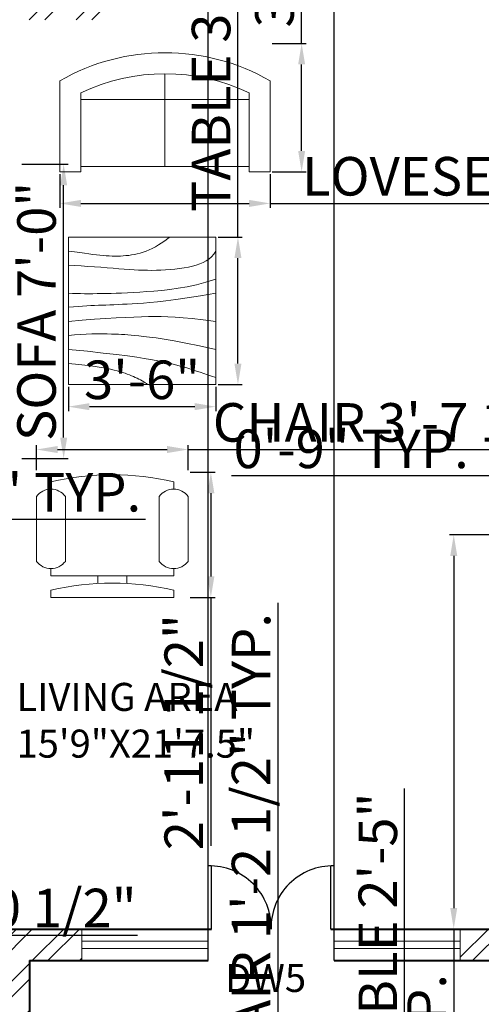
# Model space of a CAD drawing. Units: inches. Extents: x 2069 to 3028, y 691 to 1726.
# Tile 5 of 10: x 2481 to 2613, y 1044 to 1325. Entities that reach past the tile are written whole.
import ezdxf

# ---------------------------------------------------------------- set-up
doc = ezdxf.new("R2010")
doc.units = ezdxf.units.IN
for name, color, linetype, lineweight in [('A-ANNO-DIMS', 2, 'Continuous', 18), ('A-DOOR', 3, 'Continuous', 25), ('A-FURN', 8, 'Continuous', 18), ('A-GLAZ', 4, 'Continuous', 20), ('A-WALL', 7, 'Continuous', 40)]:
    doc.layers.add(name, color=color, linetype=linetype, lineweight=lineweight)
for name, color, linetype, lineweight, true_color in [('A-ANNO-TEXT', 11, 'Continuous', 18, 0xf27172), ('A-AREA-IDEN', 11, 'Continuous', 25, 0xf27172), ('A-WALL-PATT', 143, 'Continuous', 13, 0x7aafdf)]:
    doc.layers.add(name, color=color, linetype=linetype, lineweight=lineweight, true_color=true_color)
doc.styles.get("Standard").update_dxf_attribs({"font": 'arial.ttf'})
doc.dimstyles.new('ISO-25', dxfattribs={"dimtxt": 11, "dimasz": 6, "dimexe": 1.25, "dimexo": 0.625, "dimtad": 1, "dimlunit": 3, "dimtxsty": 'Standard', "dimcen": 2.5, "dimclrd": 3, "dimclre": 5, "dimclrt": 6, "dimadec": 0, "dimazin": 0, "dimtfac": 1, "dimtmove": 0, "dimatfit": 3, "dimfxl": 1, "dimarcsym": 0})

# ---------------------------------------------------------------- blocks, each defined once
blk = doc.blocks.new('Sofa - Roundback Loveseat 5 ft.')
for p, q in [((0, -32.44198), (0, -5.99998)), ((-24, -33.99998), (-24, -11.46958)), ((-23.9998, -13.38178), (23.99986, -13.38178)), ((24.00004, -33.99998), (24.00004, -11.46958)), ((-24, -32.44198), (24.00004, -32.44198))]:
    blk.add_line(p, q)
for points in [[(-24, -33.99998), (-30, -33.99998), (-30, -7.99998)], [(30.00004, -7.99998), (30.00004, -33.99998), (24.00004, -33.99998)]]:
    blk.add_lwpolyline(points)
for centre, radius, start, end in [((0, -60.24998), 60.24998, 60.13715, 119.8628), ((0, -61.38438), 55.38444, 64.32083, 115.6792)]:
    blk.add_arc(centre, radius, start, end)
blk = doc.blocks.new('Chair - Desk')
for p, q in [((-8.5, 0), (-8.5, -1)), ((-8.5, 0), (8.5, 0)), ((8.5, 0), (8.5, -1)), ((-2, -3), (-2, -1.9355)), ((2, -1.9576), (2, -3)), ((-8.5, -3), (-8.5, -4)), ((-8.5, -3), (8.5, -3)), ((8.5, -3), (8.5, -4)), ((-10.5, -5), (-10.5, -14)), ((-6.5, -14), (-6.5, -5)), ((6.5, -5), (6.5, -14)), ((10.5, -14), (10.5, -5)), ((-8.5, -15), (-8.5, -16)), ((8.5, -15), (8.5, -16))]:
    blk.add_line(p, q)
for centre, radius, start, end in [((0, 34.625), 36.625, 256.5803, 283.4197), ((-8.5, -6.5), 2.5, 36.8699, 143.1301), ((8.5, -6.5), 2.5, 36.8699, 143.1301), ((-8.5, -12.5), 2.5, 216.8699, 323.1301), ((8.5, -12.5), 2.5, 216.8699, 323.1301), ((0, 19.625), 36.625, 256.5803, 283.4197)]:
    blk.add_arc(centre, radius, start, end)
blk = doc.blocks.new('Table - Square Woodgrain 42 x 42 in.')
blk.add_line((0, -42), (42, -42))
for points in [[(0, -4), (1.704, -4.2172), (3.2358, -4.4188), (4.615, -4.604), (5.8615, -4.7721), (6.9951, -4.9224), (8.0357, -5.0541), (9.0031, -5.1667), (9.9171, -5.2594), (10.7951, -5.3316), (11.6445, -5.3836), (12.4702, -5.4157), (13.277, -5.4283), (14.0698, -5.4217), (14.8535, -5.3964), (15.6331, -5.3526), (16.4133, -5.2908), (17.1986, -5.2103), (17.9913, -5.1062), (18.793, -4.9727), (19.6056, -4.8038), (20.4307, -4.5937), (21.2701, -4.3365), (22.1256, -4.0262), (22.9989, -3.6571), (23.888, -3.2272), (24.7756, -2.7516), (25.6408, -2.2491), (26.4624, -1.7387), (27.2195, -1.2395), (27.891, -0.7703), (28.456, -0.3501), (28.8934, 0.002)], [(0, -42), (0, 0), (42, 0), (42, -42)], [(0, -8), (1.8203, -8.1001), (3.6741, -8.2149), (5.5411, -8.3408), (7.4011, -8.4741), (9.2339, -8.6112), (11.0193, -8.7484), (12.7371, -8.8821), (14.3671, -9.0086), (15.8954, -9.1246), (17.3337, -9.2278), (18.6997, -9.3159), (20.0116, -9.387), (21.2871, -9.4389), (22.5442, -9.4696), (23.8008, -9.477), (25.0749, -9.459), (26.3791, -9.4137), (27.7049, -9.3403), (29.0383, -9.2382), (30.3655, -9.1068), (31.6728, -8.9455), (32.9461, -8.7535), (34.1717, -8.5304), (35.3358, -8.2756), (36.4268, -7.9863), (37.443, -7.6521), (38.3849, -7.2603), (39.253, -6.7986), (40.048, -6.2542), (40.7705, -5.6147), (41.421, -4.8674), (42, -4)], [(42, -12), (39.1784, -12.8621), (36.4519, -13.5654), (33.8246, -14.1294), (31.3004, -14.5731), (28.8832, -14.9161), (26.577, -15.1775), (24.3858, -15.3768), (22.3136, -15.5332), (20.3622, -15.6632), (18.5254, -15.7718), (16.7947, -15.8612), (15.1618, -15.9338), (13.6183, -15.9916), (12.1558, -16.0369), (10.7659, -16.0718), (9.4403, -16.0987), (8.1703, -16.1191), (6.9461, -16.1325), (5.7577, -16.1377), (4.595, -16.1335), (3.4479, -16.1188), (2.3064, -16.0924), (1.1604, -16.0532), (0, -16)], [(42, -16), (37.6529, -16.7365), (33.8802, -17.329), (30.6179, -17.7961), (27.8015, -18.1561), (25.3668, -18.4275), (23.2497, -18.6288), (21.3859, -18.7785), (19.7111, -18.8949), (18.1693, -18.9939), (16.7375, -19.0795), (15.401, -19.1534), (14.1449, -19.217), (12.9544, -19.2717), (11.8148, -19.3191), (10.7113, -19.3606), (9.6291, -19.3976), (8.5534, -19.4323), (7.47, -19.4689), (6.3643, -19.5122), (5.222, -19.5672), (4.0288, -19.6386), (2.7703, -19.7313), (1.4321, -19.8501), (0, -20)], [(0, -24), (3.9243, -23.6805), (7.4766, -23.4138), (10.6891, -23.1954), (13.5943, -23.0205), (16.2247, -22.8847), (18.6125, -22.7832), (20.7903, -22.7116), (22.7903, -22.6651), (24.6563, -22.642), (26.4764, -22.6507), (28.35, -22.7024), (30.3766, -22.8084), (32.6555, -22.98), (35.2861, -23.2283), (38.3678, -23.5645), (42, -24)], [(42, -32), (37.392, -31.017), (33.4585, -30.2231), (30.1291, -29.5949), (27.3334, -29.109), (25.0009, -28.742), (23.0612, -28.4707), (21.4439, -28.2716), (20.0786, -28.1215), (18.8998, -28.0002), (17.8609, -27.9014), (16.9206, -27.8219), (16.0371, -27.7588), (15.1691, -27.709), (14.2748, -27.6693), (13.3128, -27.6368), (12.2415, -27.6083), (11.0295, -27.5824), (9.6867, -27.5643), (8.233, -27.5608), (6.6884, -27.5787), (5.0728, -27.6248), (3.4062, -27.7058), (1.7086, -27.8286), (0, -28)], [(0, -32), (5.4026, -32.5358), (9.9494, -33.019), (13.7424, -33.4553), (16.8834, -33.8505), (19.4743, -34.2106), (21.6171, -34.5413), (23.4136, -34.8486), (24.9657, -35.1382), (26.3614, -35.4156), (27.6332, -35.6841), (28.7995, -35.9467), (29.8788, -36.2064), (30.8897, -36.4661), (31.8507, -36.7288), (32.7802, -36.9973), (33.6968, -37.2747), (34.6175, -37.5635), (35.5531, -37.8651), (36.5128, -38.1805), (37.506, -38.5108), (38.5421, -38.8568), (39.6302, -39.2197), (40.7797, -39.6004), (42, -40)], [(0, -36), (3.0098, -36.2857), (5.5354, -36.5643), (7.6368, -36.8359), (9.374, -37.1009), (10.807, -37.3597), (11.9957, -37.6126), (13.0002, -37.8599), (13.8804, -38.102), (14.6874, -38.3393), (15.4365, -38.5729), (16.1338, -38.8041), (16.7858, -39.0341), (17.3987, -39.264), (17.9787, -39.4952), (18.5322, -39.7288), (19.0655, -39.9662), (19.5832, -40.2081), (20.0842, -40.4544), (20.5657, -40.7046), (21.0249, -40.9581), (21.459, -41.2144), (21.8653, -41.4731), (22.2409, -41.7335), (22.5831, -41.9951)]]:
    blk.add_lwpolyline(points)
blk = doc.blocks.new('*D46')
at = {"layer": 'A-ANNO-DIMS', "color": 3, "lineweight": -2, "transparency": 16777216}
for p, q in [((2554.97, 1007.13), (2554.97, 1159.02)), ((2554.97, 998.55), (2554.97, 1001.13))]:
    blk.add_line(p, q, dxfattribs=at)
at = {"layer": 'A-ANNO-DIMS', "color": 5, "lineweight": -2, "transparency": 16777216}
for p, q in [((2553.4, 1007.13), (2556.22, 1007.13)), ((2553.4, 992.55), (2556.22, 992.55))]:
    blk.add_line(p, q, dxfattribs=at)
at = {"layer": 'A-ANNO-DIMS', "color": 3, "transparency": 16777216}
for points in [[(2553.97, 1001.13), (2555.97, 1001.13), (2554.97, 1007.13)], [(2553.97, 998.55), (2555.97, 998.55), (2554.97, 992.55)]]:
    blk.add_solid(points, dxfattribs=at)
at = {"layer": 'Defpoints', "color": 0, "transparency": 16777216}
for p in [(2552.78, 1007.13), (2554.97, 1007.13), (2552.78, 992.55)]:
    blk.add_point(p, dxfattribs=at)
at = {"layer": 'A-ANNO-DIMS', "color": 6, "transparency": 16777216, "insert": (2548.65, 1086.08), "char_height": 11, "attachment_point": 5, "rotation": 90}
blk.add_mtext('CHAIR 1\'-2 1/2" TYP.', dxfattribs=at)
blk = doc.blocks.new('*D48')
at = {"layer": 'A-ANNO-DIMS', "color": 5, "lineweight": -2, "transparency": 16777216}
for p, q in [((2485.97, 1196.86), (2485.97, 1203.98)), ((2529.25, 1196.86), (2529.25, 1203.98))]:
    blk.add_line(p, q, dxfattribs=at)
at = {"layer": 'A-ANNO-DIMS', "color": 3, "lineweight": -2, "transparency": 16777216}
for p, q in [((2491.97, 1202.73), (2523.25, 1202.73)), ((2529.25, 1202.73), (2643.33, 1202.73))]:
    blk.add_line(p, q, dxfattribs=at)
at = {"layer": 'A-ANNO-DIMS', "color": 3, "transparency": 16777216}
for points in [[(2491.97, 1203.73), (2491.97, 1201.73), (2485.97, 1202.73)], [(2523.25, 1203.73), (2523.25, 1201.73), (2529.25, 1202.73)]]:
    blk.add_solid(points, dxfattribs=at)
at = {"layer": 'Defpoints', "color": 0, "transparency": 16777216}
for p in [(2529.25, 1202.73), (2485.97, 1196.23), (2529.25, 1196.23)]:
    blk.add_point(p, dxfattribs=at)
at = {"layer": 'A-ANNO-DIMS', "color": 6, "transparency": 16777216, "insert": (2589.29, 1209.04), "char_height": 11, "attachment_point": 5}
blk.add_mtext('CHAIR 3\'-7 1/2"', dxfattribs=at)
blk = doc.blocks.new('*D49')
at = {"layer": 'A-ANNO-DIMS', "color": 5, "lineweight": -2, "transparency": 16777216}
for p, q in [((2529.88, 1196.23), (2537, 1196.23)), ((2529.88, 1160.51), (2537, 1160.51))]:
    blk.add_line(p, q, dxfattribs=at)
at = {"layer": 'A-ANNO-DIMS', "color": 3, "lineweight": -2, "transparency": 16777216}
for p, q in [((2535.75, 1190.23), (2535.75, 1166.51)), ((2535.75, 1160.51), (2535.75, 1089.65))]:
    blk.add_line(p, q, dxfattribs=at)
at = {"layer": 'A-ANNO-DIMS', "color": 3, "transparency": 16777216}
for points in [[(2534.75, 1190.23), (2536.75, 1190.23), (2535.75, 1196.23)], [(2534.75, 1166.51), (2536.75, 1166.51), (2535.75, 1160.51)]]:
    blk.add_solid(points, dxfattribs=at)
at = {"layer": 'Defpoints', "color": 0, "transparency": 16777216}
for p in [(2529.25, 1196.23), (2529.25, 1160.51), (2535.75, 1160.51)]:
    blk.add_point(p, dxfattribs=at)
at = {"layer": 'A-ANNO-DIMS', "color": 6, "transparency": 16777216, "insert": (2529.43, 1122.08), "char_height": 11, "attachment_point": 5, "rotation": 90}
blk.add_mtext('2\'-11 1/2"', dxfattribs=at)
blk = doc.blocks.new('*D56')
at = {"layer": 'A-ANNO-DIMS', "color": 5, "lineweight": -2, "transparency": 16777216}
for p, q in [((2389.32, 1186.76), (2389.32, 1181.62)), ((2419.45, 1186.76), (2419.45, 1181.62))]:
    blk.add_line(p, q, dxfattribs=at)
at = {"layer": 'A-ANNO-DIMS', "color": 3, "lineweight": -2, "transparency": 16777216}
for p, q in [((2395.32, 1182.87), (2413.45, 1182.87)), ((2419.45, 1182.87), (2517.12, 1182.87))]:
    blk.add_line(p, q, dxfattribs=at)
at = {"layer": 'A-ANNO-DIMS', "color": 3, "transparency": 16777216}
for points in [[(2395.32, 1183.87), (2395.32, 1181.87), (2389.32, 1182.87)], [(2413.45, 1183.87), (2413.45, 1181.87), (2419.45, 1182.87)]]:
    blk.add_solid(points, dxfattribs=at)
at = {"layer": 'Defpoints', "color": 0, "transparency": 16777216}
for p in [(2389.32, 1187.39), (2419.45, 1187.39), (2419.45, 1182.87)]:
    blk.add_point(p, dxfattribs=at)
at = {"layer": 'A-ANNO-DIMS', "color": 6, "transparency": 16777216, "insert": (2471.28, 1189.11), "char_height": 11, "attachment_point": 5}
blk.add_mtext('D3 2\'-6" TYP.', dxfattribs=at)
blk = doc.blocks.new('*D66')
at = {"layer": 'A-ANNO-DIMS', "color": 3, "lineweight": -2, "transparency": 16777216}
for p, q in [((2591.06, 1016.25), (2591.06, 1105.97)), ((2591.06, 993.08), (2591.06, 1010.25))]:
    blk.add_line(p, q, dxfattribs=at)
at = {"layer": 'A-ANNO-DIMS', "color": 5, "lineweight": -2, "transparency": 16777216}
for p, q in [((2587.31, 1016.25), (2592.31, 1016.25)), ((2587.31, 987.08), (2592.31, 987.08))]:
    blk.add_line(p, q, dxfattribs=at)
at = {"layer": 'A-ANNO-DIMS', "color": 3, "transparency": 16777216}
for points in [[(2590.06, 1010.25), (2592.06, 1010.25), (2591.06, 1016.25)], [(2590.06, 993.08), (2592.06, 993.08), (2591.06, 987.08)]]:
    blk.add_solid(points, dxfattribs=at)
at = {"layer": 'Defpoints', "color": 0, "transparency": 16777216}
for p in [(2586.69, 1016.25), (2591.06, 1016.25), (2586.69, 987.08)]:
    blk.add_point(p, dxfattribs=at)
at = {"layer": 'A-ANNO-DIMS', "color": 6, "transparency": 16777216, "insert": (2584.82, 1064.11), "char_height": 11, "attachment_point": 5, "rotation": 90}
blk.add_mtext('TABLE 2\'-5"', dxfattribs=at)
blk = doc.blocks.new('*D68')
at = {"layer": 'A-ANNO-DIMS', "color": 3, "lineweight": -2, "transparency": 16777216}
for p, q in [((2543.48, 1263.36), (2543.48, 1353.08)), ((2543.48, 1227.27), (2543.48, 1257.36))]:
    blk.add_line(p, q, dxfattribs=at)
at = {"layer": 'A-ANNO-DIMS', "color": 5, "lineweight": -2, "transparency": 16777216}
for p, q in [((2537.79, 1263.36), (2544.73, 1263.36)), ((2537.79, 1221.27), (2544.73, 1221.27))]:
    blk.add_line(p, q, dxfattribs=at)
at = {"layer": 'A-ANNO-DIMS', "color": 3, "transparency": 16777216}
for points in [[(2542.48, 1257.36), (2544.48, 1257.36), (2543.48, 1263.36)], [(2542.48, 1227.27), (2544.48, 1227.27), (2543.48, 1221.27)]]:
    blk.add_solid(points, dxfattribs=at)
at = {"layer": 'Defpoints', "color": 0, "transparency": 16777216}
for p in [(2537.16, 1263.36), (2543.48, 1263.36), (2537.16, 1221.27)]:
    blk.add_point(p, dxfattribs=at)
at = {"layer": 'A-ANNO-DIMS', "color": 6, "transparency": 16777216, "insert": (2537.23, 1311.22), "char_height": 11, "attachment_point": 5, "rotation": 90}
blk.add_mtext('TABLE 3\'-6"', dxfattribs=at)
blk = doc.blocks.new('*D69')
at = {"layer": 'A-ANNO-DIMS', "color": 5, "lineweight": -2, "transparency": 16777216}
for p, q in [((2495.08, 1220.65), (2495.08, 1213.71)), ((2537.16, 1220.65), (2537.16, 1213.71))]:
    blk.add_line(p, q, dxfattribs=at)
at = {"layer": 'A-ANNO-DIMS', "color": 3, "lineweight": -2, "transparency": 16777216}
blk.add_line((2501.08, 1214.96), (2531.16, 1214.96), dxfattribs=at)
at = {"layer": 'A-ANNO-DIMS', "color": 3, "transparency": 16777216}
for points in [[(2501.08, 1215.96), (2501.08, 1213.96), (2495.08, 1214.96)], [(2531.16, 1215.96), (2531.16, 1213.96), (2537.16, 1214.96)]]:
    blk.add_solid(points, dxfattribs=at)
at = {"layer": 'Defpoints', "color": 0, "transparency": 16777216}
for p in [(2495.08, 1221.27), (2537.16, 1221.27), (2537.16, 1214.96)]:
    blk.add_point(p, dxfattribs=at)
at = {"layer": 'A-ANNO-DIMS', "color": 6, "transparency": 16777216, "insert": (2516.12, 1221.2), "char_height": 11, "attachment_point": 5}
blk.add_mtext('3\'-6"', dxfattribs=at)
blk = doc.blocks.new('*D72')
at = {"layer": 'A-ANNO-DIMS', "color": 5, "lineweight": -2, "transparency": 16777216}
for p, q in [((2621.33, 1178.39), (2603.83, 1178.39)), ((2621.33, 1065.89), (2603.83, 1065.89))]:
    blk.add_line(p, q, dxfattribs=at)
at = {"layer": 'A-ANNO-DIMS', "color": 3, "lineweight": -2, "transparency": 16777216}
for p, q in [((2605.08, 1172.39), (2605.08, 1071.89)), ((2605.08, 1065.89), (2605.08, 833.73))]:
    blk.add_line(p, q, dxfattribs=at)
at = {"layer": 'A-ANNO-DIMS', "color": 3, "transparency": 16777216}
for points in [[(2604.08, 1172.39), (2606.08, 1172.39), (2605.08, 1178.39)], [(2604.08, 1071.89), (2606.08, 1071.89), (2605.08, 1065.89)]]:
    blk.add_solid(points, dxfattribs=at)
at = {"layer": 'Defpoints', "color": 0, "transparency": 16777216}
for p in [(2621.95, 1178.39), (2605.08, 1065.89), (2621.95, 1065.89)]:
    blk.add_point(p, dxfattribs=at)
at = {"layer": 'A-ANNO-DIMS', "color": 6, "transparency": 16777216, "insert": (2598.76, 946.81), "char_height": 11, "attachment_point": 5, "rotation": 90}
blk.add_mtext('CASED OPENING 9\'-4 1/2" TYP.', dxfattribs=at)
blk = doc.blocks.new('*D73')
at = {"layer": 'A-ANNO-DIMS', "color": 3, "lineweight": -2, "transparency": 16777216}
for p, q in [((2615.95, 1195.26), (2541.65, 1195.26)), ((2630.95, 1195.26), (2621.95, 1195.26)), ((2636.95, 1195.26), (2642.95, 1195.26))]:
    blk.add_line(p, q, dxfattribs=at)
at = {"layer": 'A-ANNO-DIMS', "color": 5, "lineweight": -2, "transparency": 16777216}
for p, q in [((2621.95, 1179.01), (2621.95, 1196.51)), ((2630.95, 1179.01), (2630.95, 1196.51))]:
    blk.add_line(p, q, dxfattribs=at)
at = {"layer": 'A-ANNO-DIMS', "color": 3, "transparency": 16777216}
for points in [[(2615.95, 1196.26), (2615.95, 1194.26), (2621.95, 1195.26)], [(2636.95, 1196.26), (2636.95, 1194.26), (2630.95, 1195.26)]]:
    blk.add_solid(points, dxfattribs=at)
at = {"layer": 'Defpoints', "color": 0, "transparency": 16777216}
for p in [(2621.95, 1195.26), (2621.95, 1178.39), (2630.95, 1178.39)]:
    blk.add_point(p, dxfattribs=at)
at = {"layer": 'A-ANNO-DIMS', "color": 6, "transparency": 16777216, "insert": (2575.8, 1201.5), "char_height": 11, "attachment_point": 5}
blk.add_mtext('0\'-9" TYP.', dxfattribs=at)
blk = doc.blocks.new('*D76')
at = {"layer": 'A-ANNO-DIMS', "color": 5, "lineweight": -2, "transparency": 16777216}
for p, q in [((2378.21, 1067.22), (2378.21, 1062.91)), ((2402.76, 1067.22), (2402.76, 1062.91))]:
    blk.add_line(p, q, dxfattribs=at)
at = {"layer": 'A-ANNO-DIMS', "color": 3, "lineweight": -2, "transparency": 16777216}
for p, q in [((2384.21, 1064.16), (2396.76, 1064.16)), ((2402.76, 1064.16), (2514.78, 1064.16))]:
    blk.add_line(p, q, dxfattribs=at)
at = {"layer": 'A-ANNO-DIMS', "color": 3, "transparency": 16777216}
for points in [[(2384.21, 1065.16), (2384.21, 1063.16), (2378.21, 1064.16)], [(2396.76, 1065.16), (2396.76, 1063.16), (2402.76, 1064.16)]]:
    blk.add_solid(points, dxfattribs=at)
at = {"layer": 'Defpoints', "color": 0, "transparency": 16777216}
for p in [(2378.21, 1067.84), (2402.76, 1067.84), (2402.76, 1064.16)]:
    blk.add_point(p, dxfattribs=at)
at = {"layer": 'A-ANNO-DIMS', "color": 6, "transparency": 16777216, "insert": (2461.77, 1070.47), "char_height": 11, "attachment_point": 5}
blk.add_mtext('BASIN 2\'-0 1/2"', dxfattribs=at)
blk = doc.blocks.new('*D80')
at = {"layer": 'A-ANNO-DIMS', "color": 5, "lineweight": -2, "transparency": 16777216}
for p, q in [((2492.66, 1281.34), (2492.66, 1271.71)), ((2552.66, 1281.34), (2552.66, 1271.71))]:
    blk.add_line(p, q, dxfattribs=at)
at = {"layer": 'A-ANNO-DIMS', "color": 3, "lineweight": -2, "transparency": 16777216}
for p, q in [((2498.66, 1272.96), (2546.66, 1272.96)), ((2552.66, 1272.96), (2674.06, 1272.96))]:
    blk.add_line(p, q, dxfattribs=at)
at = {"layer": 'A-ANNO-DIMS', "color": 3, "transparency": 16777216}
for points in [[(2498.66, 1273.96), (2498.66, 1271.96), (2492.66, 1272.96)], [(2546.66, 1273.96), (2546.66, 1271.96), (2552.66, 1272.96)]]:
    blk.add_solid(points, dxfattribs=at)
at = {"layer": 'Defpoints', "color": 0, "transparency": 16777216}
for p in [(2492.66, 1281.96), (2552.66, 1281.96), (2552.66, 1272.96)]:
    blk.add_point(p, dxfattribs=at)
at = {"layer": 'A-ANNO-DIMS', "color": 6, "transparency": 16777216, "insert": (2616.36, 1279.28), "char_height": 11, "attachment_point": 5}
blk.add_mtext('LOVESEAT 5\'-0"', dxfattribs=at)
blk = doc.blocks.new('*D81')
at = {"layer": 'A-ANNO-DIMS', "color": 3, "lineweight": -2, "transparency": 16777216}
for p, q in [((2561.66, 1318.63), (2561.66, 1380.74)), ((2561.66, 1287.96), (2561.66, 1312.63))]:
    blk.add_line(p, q, dxfattribs=at)
at = {"layer": 'A-ANNO-DIMS', "color": 5, "lineweight": -2, "transparency": 16777216}
for p, q in [((2553.28, 1318.63), (2562.91, 1318.63)), ((2553.28, 1281.96), (2562.91, 1281.96))]:
    blk.add_line(p, q, dxfattribs=at)
at = {"layer": 'A-ANNO-DIMS', "color": 3, "transparency": 16777216}
for points in [[(2560.66, 1312.63), (2562.66, 1312.63), (2561.66, 1318.63)], [(2560.66, 1287.96), (2562.66, 1287.96), (2561.66, 1281.96)]]:
    blk.add_solid(points, dxfattribs=at)
at = {"layer": 'Defpoints', "color": 0, "transparency": 16777216}
for p in [(2552.66, 1318.63), (2561.66, 1318.63), (2552.66, 1281.96)]:
    blk.add_point(p, dxfattribs=at)
at = {"layer": 'A-ANNO-DIMS', "color": 6, "transparency": 16777216, "insert": (2555.34, 1352.69), "char_height": 11, "attachment_point": 5, "rotation": 90}
blk.add_mtext('3\'-0 1/2"', dxfattribs=at)
blk = doc.blocks.new('*D82')
at = {"layer": 'A-ANNO-DIMS', "color": 5, "lineweight": -2, "transparency": 16777216}
for p, q in [((2481.75, 1284.15), (2494.98, 1284.15)), ((2481.75, 1200.15), (2494.98, 1200.15))]:
    blk.add_line(p, q, dxfattribs=at)
at = {"layer": 'A-ANNO-DIMS', "color": 3, "lineweight": -2, "transparency": 16777216}
blk.add_line((2493.73, 1206.15), (2493.73, 1278.15), dxfattribs=at)
at = {"layer": 'A-ANNO-DIMS', "color": 3, "transparency": 16777216}
for points in [[(2492.73, 1278.15), (2494.73, 1278.15), (2493.73, 1284.15)], [(2492.73, 1206.15), (2494.73, 1206.15), (2493.73, 1200.15)]]:
    blk.add_solid(points, dxfattribs=at)
at = {"layer": 'Defpoints', "color": 0, "transparency": 16777216}
for p in [(2481.13, 1284.15), (2493.73, 1284.15), (2481.13, 1200.15)]:
    blk.add_point(p, dxfattribs=at)
at = {"layer": 'A-ANNO-DIMS', "color": 6, "transparency": 16777216, "insert": (2487.41, 1242.15), "char_height": 11, "attachment_point": 5, "rotation": 90}
blk.add_mtext('SOFA 7\'-0"', dxfattribs=at)
blk = doc.blocks.new('*D89')
at = {"layer": 'A-ANNO-DIMS', "color": 5, "lineweight": -2, "transparency": 16777216}
for p, q in [((2336.92, 747.01), (2336.92, 1704.14)), ((2711.95, 747.01), (2711.95, 1704.14))]:
    blk.add_line(p, q, dxfattribs=at)
at = {"layer": 'A-ANNO-DIMS', "color": 3, "lineweight": -2, "transparency": 16777216}
blk.add_line((2342.92, 1702.89), (2705.95, 1702.89), dxfattribs=at)
at = {"layer": 'A-ANNO-DIMS', "color": 3, "transparency": 16777216}
for points in [[(2342.92, 1703.89), (2342.92, 1701.89), (2336.92, 1702.89)], [(2705.95, 1703.89), (2705.95, 1701.89), (2711.95, 1702.89)]]:
    blk.add_solid(points, dxfattribs=at)
at = {"layer": 'Defpoints', "color": 0, "transparency": 16777216}
for p in [(2711.95, 1702.89), (2336.92, 746.39), (2711.95, 746.39)]:
    blk.add_point(p, dxfattribs=at)
at = {"layer": 'A-ANNO-DIMS', "color": 6, "transparency": 16777216, "insert": (2524.44, 1709.13), "char_height": 11, "attachment_point": 5}
blk.add_mtext('31\'-3"', dxfattribs=at)
blk = doc.blocks.new('*D96')
at = {"layer": 'A-ANNO-DIMS', "color": 5, "lineweight": -2, "transparency": 16777216}
for p, q in [((2534.95, 1066.51), (2534.95, 1704.14)), ((2570.95, 1066.51), (2570.95, 1704.14))]:
    blk.add_line(p, q, dxfattribs=at)
at = {"layer": 'A-ANNO-DIMS', "color": 3, "lineweight": -2, "transparency": 16777216}
blk.add_line((2540.95, 1702.89), (2564.95, 1702.89), dxfattribs=at)
at = {"layer": 'A-ANNO-DIMS', "color": 3, "transparency": 16777216}
for points in [[(2540.95, 1703.89), (2540.95, 1701.89), (2534.95, 1702.89)], [(2564.95, 1703.89), (2564.95, 1701.89), (2570.95, 1702.89)]]:
    blk.add_solid(points, dxfattribs=at)
at = {"layer": 'Defpoints', "color": 0, "transparency": 16777216}
for p in [(2570.95, 1702.89), (2534.95, 1065.89), (2570.95, 1065.89)]:
    blk.add_point(p, dxfattribs=at)
at = {"layer": 'A-ANNO-DIMS', "color": 6, "transparency": 16777216, "insert": (2552.95, 1709.13), "char_height": 11, "attachment_point": 5}
blk.add_mtext('3\'-0"', dxfattribs=at)

msp = doc.modelspace()

# ---------------------------------------------------------------- hatches: boundary and pattern name
at = {"layer": 'A-WALL-PATT'}
h = msp.add_hatch(dxfattribs=at)
h.set_pattern_fill('ANSI32', color=256)
h.paths.add_polyline_path([(2675.951, 1487.387), (2576.951, 1487.387), (2576.951, 1478.387), (2621.951, 1478.387), (2621.951, 1365.287), (2630.951, 1365.287), (2630.951, 1478.387), (2675.951, 1478.387)])
h.paths.add_polyline_path([(2765.951, 1487.387), (2711.951, 1487.387), (2711.951, 1478.387), (2756.951, 1478.387), (2756.951, 1424.387), (2765.951, 1424.387)])
h.paths.add_polyline_path([(2528.951, 1487.387), (2407.751, 1487.387), (2407.751, 1478.387), (2474.951, 1478.387), (2474.951, 1434.887), (2498.951, 1434.887), (2498.951, 1374.887), (2474.951, 1374.887), (2474.951, 1365.287), (2483.951, 1365.287), (2483.951, 1370.387), (2507.951, 1370.387), (2507.951, 1439.387), (2483.951, 1439.387), (2483.951, 1478.387), (2528.951, 1478.387)])
h.paths.add_polyline_path([(2374.151, 1487.387), (2297.951, 1487.387), (2297.951, 1424.387), (2306.951, 1424.387), (2306.951, 1478.387), (2374.151, 1478.387)])
h.paths.add_polyline_path([(2507.951, 1334.387), (2483.951, 1334.387), (2483.951, 1338.887), (2474.951, 1338.887), (2474.951, 1334.387), (2306.951, 1334.387), (2306.951, 1388.387), (2297.951, 1388.387), (2297.951, 1334.387), (2267.951, 1334.387), (2267.951, 1274.387), (2276.951, 1274.387), (2276.951, 1325.387), (2297.951, 1325.387), (2423.951, 1325.387), (2423.951, 1187.387), (2419.451, 1187.387), (2419.451, 1178.387), (2432.951, 1178.387), (2432.951, 1325.387), (2507.951, 1325.387)])
h.paths.add_polyline_path([(2795.951, 1334.387), (2630.951, 1334.387), (2630.951, 1338.887), (2621.951, 1338.887), (2621.951, 1178.387), (2635.451, 1178.387), (2635.451, 1187.387), (2630.951, 1187.387), (2630.951, 1325.387), (2786.951, 1325.387), (2786.951, 1274.387), (2795.951, 1274.387)])
h.paths.add_polyline_path([(2765.951, 1388.387), (2756.951, 1388.387), (2756.951, 1334.387), (2765.951, 1334.387)])
h.paths.add_polyline_path([(2795.951, 1238.387), (2786.951, 1238.387), (2786.951, 1187.387), (2665.451, 1187.387), (2665.451, 1178.387), (2795.951, 1178.387)], flags=17)
h.paths.add_polyline_path([(2389.451, 1187.387), (2276.951, 1187.387), (2276.951, 1238.387), (2267.951, 1238.387), (2267.951, 1178.387), (2297.951, 1178.387), (2297.951, 1173.287), (2307.451, 1173.287), (2307.451, 1178.387), (2389.451, 1178.387)])
h.paths.add_polyline_path([(2377.451, 1142.387), (2306.951, 1142.387), (2306.951, 1146.887), (2297.951, 1146.887), (2297.951, 1142.387), (2297.951, 1137.887), (2306.951, 1137.887), (2372.951, 1137.887), (2372.951, 1133.387), (2377.451, 1133.387)])
h.paths.add_polyline_path([(2795.951, 1065.887), (2665.451, 1065.887), (2665.451, 1056.887), (2786.951, 1056.887), (2786.951, 1002.887), (2795.951, 1002.887), (2795.951, 1056.887)])
h.paths.add_polyline_path([(2795.951, 966.887), (2786.951, 966.887), (2786.951, 912.887), (2732.951, 912.887), (2732.951, 903.887), (2795.951, 903.887)])
h.paths.add_polyline_path([(2483.951, 917.387), (2474.951, 917.387), (2474.951, 912.887), (2414.951, 912.887), (2414.951, 903.887), (2483.951, 903.887)])
h.paths.add_polyline_path([(2366.951, 912.887), (2306.951, 912.887), (2306.951, 960.887), (2297.951, 960.887), (2297.951, 903.887), (2366.951, 903.887)])
h.paths.add_polyline_path([(2498.951, 1056.887), (2498.951, 1065.887), (2377.451, 1065.887), (2377.451, 1111.787), (2372.951, 1111.787), (2372.951, 1065.887), (2306.951, 1065.887), (2306.951, 1116.287), (2297.951, 1116.287), (2297.951, 1056.887), (2297.951, 1008.887), (2306.951, 1008.887), (2306.951, 1056.887), (2474.951, 1056.887), (2474.951, 947.387), (2483.951, 947.387), (2483.951, 1056.887)])
h = msp.add_hatch(dxfattribs=at)
h.set_pattern_fill('ANSI32', color=256)
h.paths.add_polyline_path([(2684.951, 912.887), (2630.951, 912.887), (2630.951, 1056.887), (2635.451, 1056.887), (2635.451, 1065.887), (2606.951, 1065.887), (2606.951, 1056.887), (2621.951, 1056.887), (2621.951, 903.887), (2684.951, 903.887)])

# ---------------------------------------------------------------- linework, layer by layer
at = {"layer": 'A-DOOR'}
for p, q in [((2534.951, 1065.887), (2534.951, 1083.887)), ((2535.951, 1065.887), (2535.951, 1083.887)), ((2569.951, 1065.887), (2569.951, 1083.887)), ((2570.951, 1065.887), (2570.951, 1083.887)), ((2534.951, 1056.887), (2534.951, 1065.887)), ((2570.951, 1056.887), (2570.951, 1065.887))]:
    msp.add_line(p, q, dxfattribs=at)
for centre, start, end in [((2535.451, 1066.387), 358.36342, 91.63658), ((2570.451, 1066.387), 88.36342, 181.63658)]:
    msp.add_arc(centre, 17.507, start, end, dxfattribs=at)
at = {"layer": 'A-GLAZ'}
for p, q in [((2498.951, 1056.887), (2498.951, 1065.887)), ((2606.951, 1056.887), (2606.951, 1065.887)), ((2498.951, 1062.387), (2534.951, 1062.387)), ((2498.951, 1062.387), (2534.951, 1062.387)), ((2570.951, 1062.387), (2606.951, 1062.387)), ((2570.951, 1062.387), (2606.951, 1062.387)), ((2498.951, 1060.387), (2534.951, 1060.387)), ((2570.951, 1060.387), (2606.951, 1060.387))]:
    msp.add_line(p, q, dxfattribs=at)
at = {"layer": 'A-WALL'}
for p, q in [((2377.451, 1065.887), (2535.951, 1065.887)), ((2569.951, 1065.887), (2635.451, 1065.887)), ((2483.951, 1056.887), (2483.951, 947.387)), ((2483.951, 1056.887), (2534.951, 1056.887)), ((2570.951, 1056.887), (2621.951, 1056.887))]:
    msp.add_line(p, q, dxfattribs=at)

# ---------------------------------------------------------------- block references
at = {"layer": 'A-FURN'}
msp.add_blockref('Sofa - Roundback Loveseat 5 ft.', (2522.655, 1315.963), dxfattribs=at)
at = {"layer": 'A-FURN', "xscale": 1.002105598790615, "yscale": 1.002105598790615, "zscale": 1.002105598790615}
msp.add_blockref('Table - Square Woodgrain 42 x 42 in.', (2495.075, 1263.359), dxfattribs=at)
at = {"layer": 'A-FURN', "xscale": -2.061190718686809, "yscale": 2.061190718686809, "zscale": 2.061190718686809, "rotation": 180}
msp.add_blockref('Chair - Desk', (2507.611, 1160.507), dxfattribs=at)

# ---------------------------------------------------------------- texts
at = {"layer": 'A-ANNO-TEXT', "insert": (2539.789, 1055.934), "char_height": 8, "attachment_point": 1}
msp.add_mtext_dynamic_manual_height_columns('{\\fArial|b1|i0|c0|p34;DW5}', width=34.05605, gutter_width=12.5, heights=[0], dxfattribs=at)
at = {"layer": 'A-AREA-IDEN', "insert": (2480.265, 1136.139), "char_height": 8, "attachment_point": 1}
msp.add_mtext_dynamic_manual_height_columns('LIVING AREA\\P15\'9"X21\'7.5"', width=119.20948, gutter_width=12.5, heights=[0], dxfattribs=at)

# ---------------------------------------------------------------- dimensions: what is measured, and where the dimension line sits
at = {"layer": 'A-ANNO-DIMS'}
for base, p1, p2, picture, middle in [((2711.951, 1702.887), (2336.919, 746.387), (2711.951, 746.387), '*D89', (2524.435, 1709.132)), ((2570.951, 1702.887), (2534.951, 1065.887), (2570.951, 1065.887), '*D96', (2552.951, 1709.132)), ((2537.164, 1214.957), (2495.075, 1221.271), (2537.164, 1221.271), '*D69', (2516.12, 1221.202))]:
    dim = msp.add_linear_dim(base=base, p1=p1, p2=p2, dimstyle='ISO-25', override={"dimdec": 1, "dimlfac": 1, "dimrnd": 0, "dimzin": 1, "dimdsep": 46, "dimlunit": 4, "dimfrac": 2}, dxfattribs=at)
    dim.commit()
    dim.dimension.update_dxf_attribs({"geometry": picture, "text_midpoint": middle})
for base, p1, p2, angle, picture, middle in [((2561.655, 1318.63), (2552.655, 1281.963), (2552.655, 1318.63), 90, '*D81', (2555.339, 1352.687)), ((2535.746, 1160.507), (2529.253, 1196.234), (2529.253, 1160.507), 270, '*D49', (2529.434, 1122.079))]:
    dim = msp.add_linear_dim(base=base, p1=p1, p2=p2, angle=angle, dimstyle='ISO-25', override={"dimdec": 1, "dimlfac": 1, "dimrnd": 0, "dimzin": 1, "dimdsep": 46, "dimlunit": 4, "dimfrac": 2}, dxfattribs=at)
    dim.commit()
    dim.dimension.update_dxf_attribs({"geometry": picture, "text_midpoint": middle})
for base, p1, p2, angle, text, picture, middle in [((2543.478, 1263.361), (2537.164, 1221.271), (2537.164, 1263.361), 90, 'TABLE <>', '*D68', (2537.232, 1311.221)), ((2493.726, 1284.149), (2481.126, 1200.149), (2481.126, 1284.149), 90, 'SOFA <>', '*D82', (2487.409, 1242.149)), ((2621.951, 1195.262), (2630.951, 1178.387), (2621.951, 1178.387), 180, '<> TYP.', '*D73', (2575.801, 1201.503)), ((2605.076, 1065.887), (2621.951, 1178.387), (2621.951, 1065.887), 270, 'CASED OPENING <> TYP.', '*D72', (2598.76, 946.808)), ((2554.965, 1007.135), (2552.778, 992.55), (2552.778, 1007.135), 90, 'CHAIR <> TYP.', '*D46', (2548.653, 1086.078)), ((2591.061, 1016.25), (2586.686, 987.079), (2586.686, 1016.25), 90, 'TABLE <>', '*D66', (2584.82, 1064.11))]:
    dim = msp.add_linear_dim(base=base, p1=p1, p2=p2, angle=angle, text=text, dimstyle='ISO-25', override={"dimdec": 1, "dimlfac": 1, "dimrnd": 0, "dimzin": 1, "dimdsep": 46, "dimlunit": 4, "dimfrac": 2}, dxfattribs=at)
    dim.commit()
    dim.dimension.update_dxf_attribs({"geometry": picture, "text_midpoint": middle})
for base, p1, p2, text, picture, middle in [((2552.655, 1272.963), (2492.655, 1281.963), (2552.655, 1281.963), 'LOVESEAT <>', '*D80', (2616.359, 1279.28)), ((2529.253, 1202.727), (2485.968, 1196.234), (2529.253, 1196.234), 'CHAIR <>', '*D48', (2589.291, 1209.043)), ((2419.451, 1182.866), (2389.316, 1187.387), (2419.451, 1187.387), 'D3 <> TYP.', '*D56', (2471.284, 1189.111)), ((2402.7574, 1064.1609), (2378.2065, 1067.8435), (2402.7574, 1067.8435), 'BASIN <>', '*D76', (2461.7675, 1070.4735))]:
    dim = msp.add_linear_dim(base=base, p1=p1, p2=p2, text=text, dimstyle='ISO-25', override={"dimdec": 1, "dimlfac": 1, "dimrnd": 0, "dimzin": 1, "dimdsep": 46, "dimlunit": 4, "dimfrac": 2}, dxfattribs=at)
    dim.commit()
    dim.dimension.update_dxf_attribs({"geometry": picture, "text_midpoint": middle})

doc.saveas('drawing.dxf')
